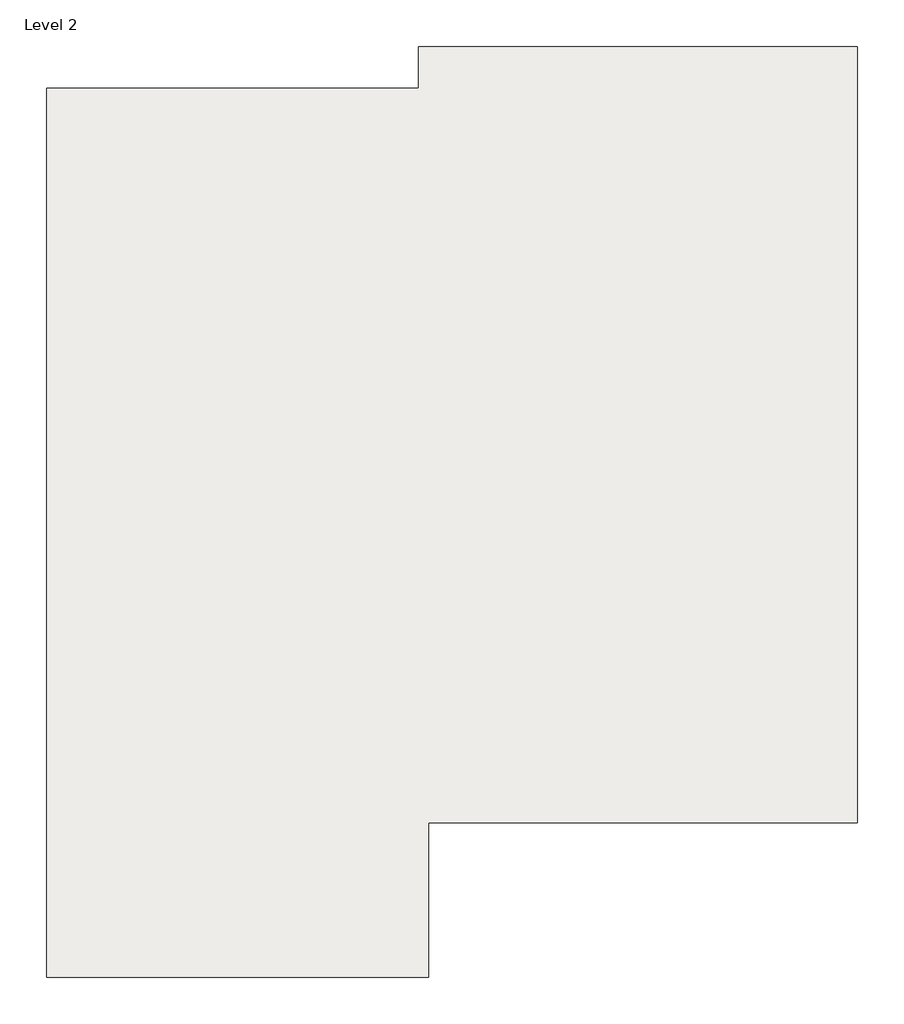
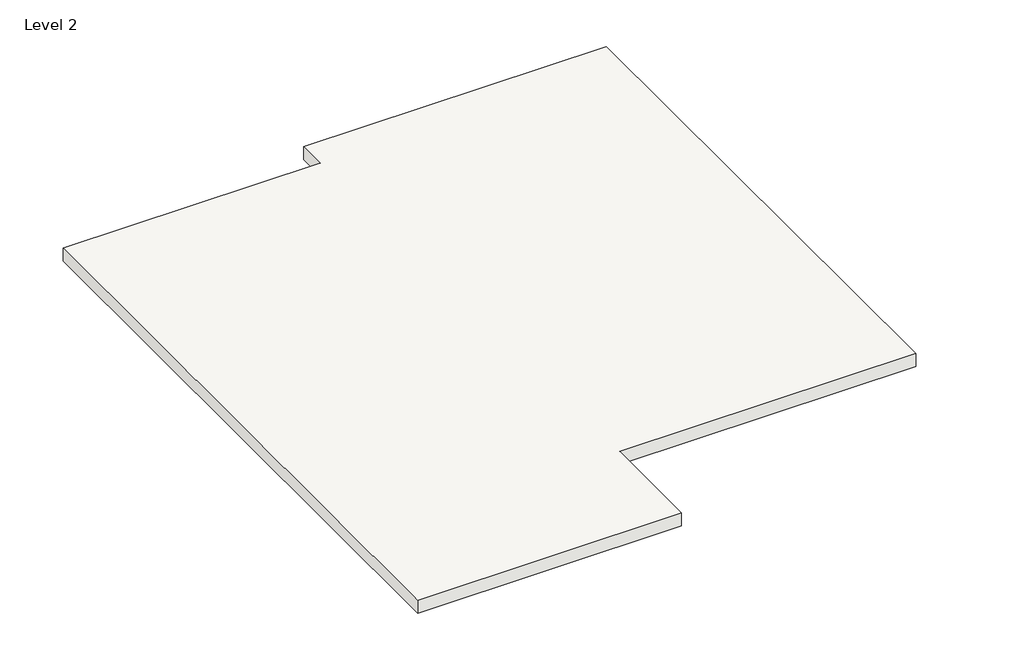
# One storey: 1 roof.
"""IFC4 building model written with IfcOpenShell, lengths in millimetres."""

from ifc_helpers import new_model, si_unit, frame, origin, place, context, project, spatial, polyline, outline, extrude, element, save

model = new_model("IFC4")

# Units and contexts
model_context = context("Model", 3, world=origin())
ifc_project = project(units=[si_unit("LENGTHUNIT", "METRE", prefix="MILLI")], contexts=[model_context])

# Site, building, storey
site = spatial("IfcSite", under=ifc_project)
building = spatial("IfcBuilding", under=site)
storey = spatial("IfcBuildingStorey", under=building, Name="Level 2", Elevation=3048.0)

# Roof
placement = place(None, origin())
element("IfcRoof", 1, ObjectType="Generic - 12\"", at=placement, inside=storey, context=model_context, shape_type="SweptSolid", body=[
    extrude(outline(polyline([(-6254.9254147, 10432.1742707), (-565.3254147, 10432.1742707), (-565.3254147, 11067.1742707), (6140.2745853, 11067.1742707), (6140.2745853, -794.6257293), (-412.9254147, -794.6257293), (-412.9254147, -3156.8257293), (-6254.9254147, -3156.8257293), (-6254.9254147, 10432.1742707)])), frame((0.0, 0.0, 3048.0), z_axis=(0.0, 0.0, 1.0), x_axis=(1.0, 0.0, 0.0)), (0.0, 0.0, 1.0), 304.8),
])

save(model, "model.ifc")

# Revit data of these elements
# Type "Generic - 12\""
#   Assembly Code = "B1020"
#   Layers, outside or top first: 1' - 0" "Brick, Soldier Course" (function 1)
# Element 1 (IfcRoof, "Generic - 12\"")
#   built-in parameter 1001705 = 11 (stored number, unit not read)
#   built-in parameter 1001710 = 33615
#   Phase Created = New Construction
#   Materials on its faces: "Brick, Soldier Course"
# Materials
#   "Brick, Soldier Course": class "Masonry", colour RGB 170 98 104, transparency 0, Description = "Common brick soldier coursed", Cost = 0
